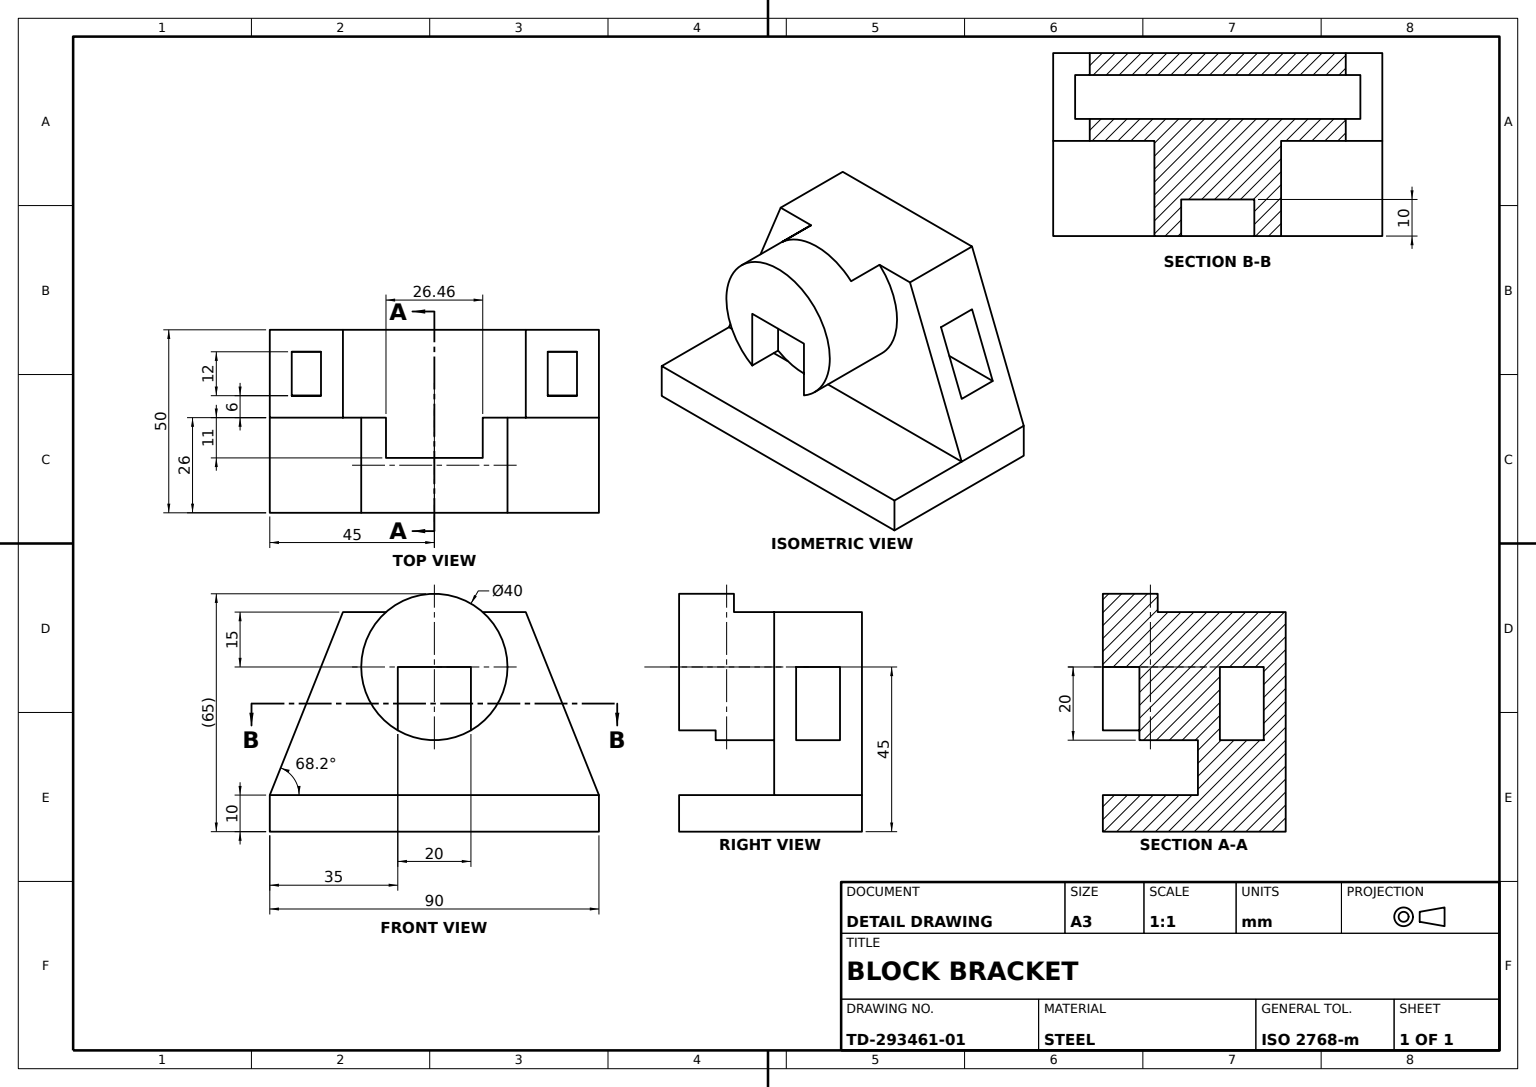
from build123d import *

# Parameters (mm, degrees)
BASE_PLATE_SKETCH_W       = 50
BASE_PLATE_SKETCH_H       = 90
BASE_PLATE_90X50X10_DEPTH = 10
UPRIGHT_WEB_DEPTH         = 24
WEB_WINDOW_CUT_DEPTH      = 112.018016556
WEB_WINDOW_CUT_DEPTH_BACK = 100
WEB_WINDOW_SKETCH_W       = 12
WEB_WINDOW_SKETCH_H       = 20
CYLINDER_BOSS_SKETCH_R    = 20
CYLINDER_BOSS_DEPTH       = 26
BOSS_START                = -10
BOSS_END_SLOT_20X10_DEPTH = 10
TOP_NOTCH_CUT_DEPTH       = 11


with BuildPart() as part:
    # Base Plate Sketch → Base Plate 90x50x10 (new body)
    with BuildSketch(Plane(origin=(0, 0, 0), x_dir=(1, 0, 0), z_dir=(0, 1, 0))):
        Rectangle(BASE_PLATE_SKETCH_W, BASE_PLATE_SKETCH_H)
    extrude(amount=BASE_PLATE_90X50X10_DEPTH)

    # Upright Web Sketch → Upright Web (add)
    with BuildSketch(Plane.ZY.offset(25)):
        Polygon((-25, 60), (25, 60), (45, 10), (-45, 10), align=None)
    extrude(amount=-UPRIGHT_WEB_DEPTH)

    # Web Window Sketch → Web Window Cut (cut, two sides: drawn at the far end of the back side and taken through both)
    with BuildSketch(Plane(origin=(0, 0, -45), x_dir=(-1, 0, 0), z_dir=(0, 0, -1)).offset(-WEB_WINDOW_CUT_DEPTH_BACK)):
        with Locations((13, 35)):
            Rectangle(WEB_WINDOW_SKETCH_W, WEB_WINDOW_SKETCH_H)
    extrude(amount=WEB_WINDOW_CUT_DEPTH + WEB_WINDOW_CUT_DEPTH_BACK, mode=Mode.SUBTRACT)

    # Cylinder Boss Sketch → Cylinder Boss (add)
    with BuildSketch(Plane(origin=(-1, 0, 0), x_dir=(0, 0, -1), z_dir=(1, 0, 0))):
        with Locations(Location((0, 45, 0), (0, 0, 131.409622109))):
            Circle(CYLINDER_BOSS_SKETCH_R)
    extrude(amount=CYLINDER_BOSS_DEPTH)

    # Boss End Slot Sketch → Boss End Slot 20x10 (cut)
    with BuildSketch(Plane(origin=(25, 0, 0), x_dir=(0, 0, -1), z_dir=(1, 0, 0)).offset(BOSS_START)):
        with BuildLine():
            Line((-10, 45), (10, 45))
            Line((10, 45), (10, 27.679491924))
            ThreePointArc((10, 27.679491924), (0, 25), (-10, 27.679491924))
            Line((-10, 27.679491924), (-10, 45))
        make_face()
    extrude(amount=BOSS_END_SLOT_20X10_DEPTH, mode=Mode.SUBTRACT)

    # Top Notch Sketch → Top Notch Cut (cut)
    with BuildSketch(Plane.ZY.offset(1)):
        with BuildLine():
            Line((-13.228756555, 60), (13.228756555, 60))
            ThreePointArc((13.228756555, 60), (0, 65), (-13.228756555, 60))
        make_face()
    extrude(amount=-TOP_NOTCH_CUT_DEPTH, mode=Mode.SUBTRACT)


solid = part.part
